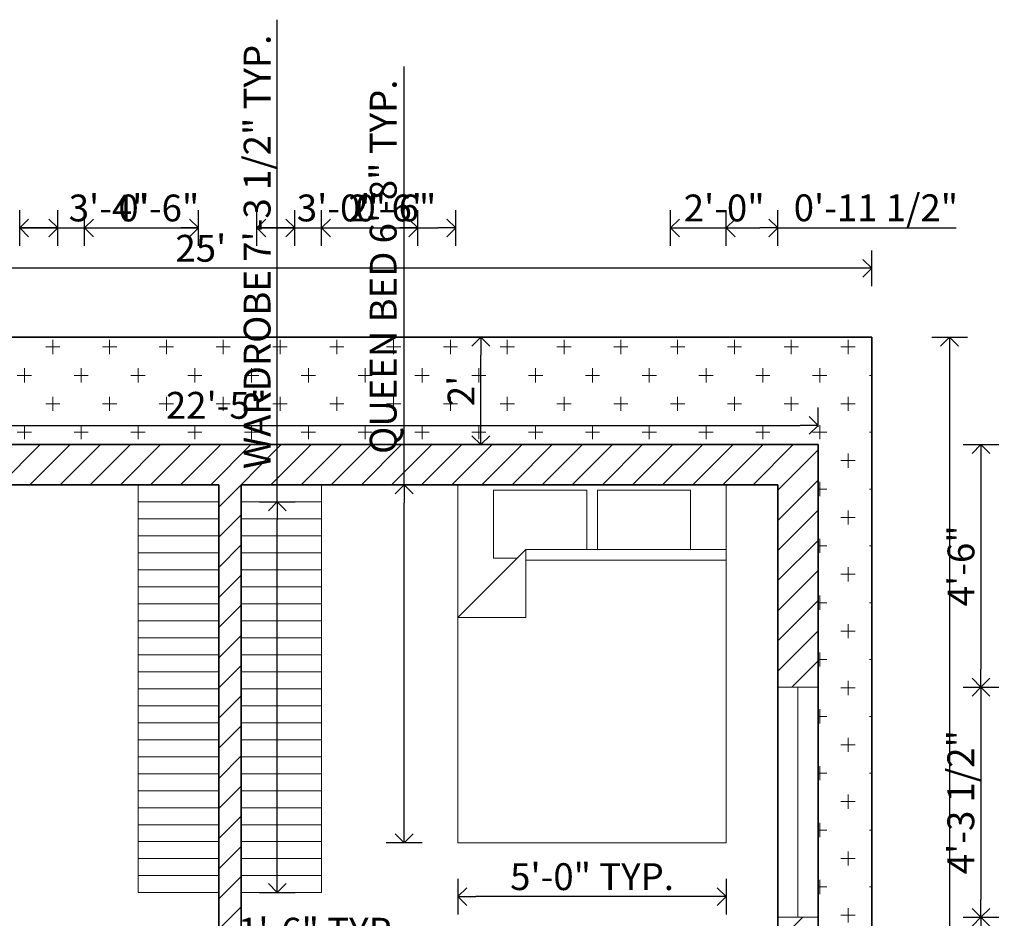
# Model space of a CAD drawing. Units: inches. Extents: x 686 to 1065, y 83 to 664.
# Tile 5 of 5: x 833 to 1053, y 463 to 664. Entities that reach past the tile are written whole.
import ezdxf

# ---------------------------------------------------------------- set-up
doc = ezdxf.new("R2010")
doc.units = ezdxf.units.IN
for name, color, linetype, lineweight in [('A-ANNO-DIMS', 2, 'Continuous', 18), ('A-FLOR-CABN', 8, 'Continuous', 20), ('A-FURN', 8, 'Continuous', 18), ('A-GLAZ', 172, 'Continuous', 18), ('A-WALL', 7, 'Continuous', 35), ('A-WALL-PATT', 253, 'Continuous', 13), ('C-PROP', 7, 'Continuous', 35), ('L-SITE-PATT', 94, 'Continuous', 13)]:
    doc.layers.add(name, color=color, linetype=linetype, lineweight=lineweight)
doc.styles.get("Standard").update_dxf_attribs({"font": 'arial.ttf'})
doc.dimstyles.new('ISO-25', dxfattribs={"dimtxt": 6, "dimasz": 4, "dimexe": 4, "dimexo": 4, "dimtad": 1, "dimdec": 1, "dimlunit": 3, "dimtxsty": 'Standard', "dimblk": 'OPEN90', "dimcen": 2.5, "dimadec": 0, "dimazin": 0, "dimtfac": 1, "dimtdec": 1, "dimtmove": 0, "dimatfit": 3, "dimfxl": 4, "dimfxlon": 1, "dimarcsym": 0})

# ---------------------------------------------------------------- blocks, each defined once
blk = doc.blocks.new('_Open90')
at = {"color": 0, "linetype": 'ByBlock', "lineweight": -2}
for p, q in [((0, 0), (-1, 0)), ((-0.5, 0.5), (0, 0)), ((0, 0), (-0.5, -0.5))]:
    blk.add_line(p, q, dxfattribs=at)
blk = doc.blocks.new('*D10')
at = {"layer": 'A-ANNO-DIMS', "color": 0, "lineweight": -2, "transparency": 16777216}
for p, q in [((939.95, 592.73), (931.95, 592.73)), ((935.95, 572.73), (935.95, 588.73)), ((939.95, 568.73), (931.95, 568.73))]:
    blk.add_line(p, q, dxfattribs=at)
at = {"layer": 'Defpoints', "color": 0, "transparency": 16777216}
for p in [(935.95, 592.73), (1011.37, 592.73), (1011.37, 568.73)]:
    blk.add_point(p, dxfattribs=at)
at = {"layer": 'A-ANNO-DIMS', "color": 0, "lineweight": -2, "transparency": 16777216, "xscale": 4, "yscale": 4, "zscale": 4}
for p, rotation in [((935.95, 592.73), 90), ((935.95, 568.73), 270)]:
    blk.add_blockref('_Open90', p, dxfattribs=dict(at, rotation=rotation))
at = {"layer": 'A-ANNO-DIMS', "color": 0, "transparency": 16777216, "insert": (932.32, 580.73), "char_height": 6, "attachment_point": 5, "rotation": 90}
blk.add_mtext("2'", dxfattribs=at)
blk = doc.blocks.new('*D11')
at = {"layer": 'A-ANNO-DIMS', "color": 0, "lineweight": -2, "transparency": 16777216}
for p, q in [((742.37, 572.73), (742.37, 577.04)), ((1011.37, 572.73), (1011.37, 577.04)), ((746.37, 573.04), (1007.37, 573.04))]:
    blk.add_line(p, q, dxfattribs=at)
at = {"layer": 'Defpoints', "color": 0, "transparency": 16777216}
for p in [(1011.37, 573.04), (742.37, 568.73), (1011.37, 568.73)]:
    blk.add_point(p, dxfattribs=at)
at = {"layer": 'A-ANNO-DIMS', "color": 0, "lineweight": -2, "transparency": 16777216, "xscale": 4, "yscale": 4, "zscale": 4, "rotation": 180}
blk.add_blockref('_Open90', (742.37, 573.04), dxfattribs=at)
at = {"layer": 'A-ANNO-DIMS', "color": 0, "lineweight": -2, "transparency": 16777216, "xscale": 4, "yscale": 4, "zscale": 4}
blk.add_blockref('_Open90', (1011.37, 573.04), dxfattribs=at)
at = {"layer": 'A-ANNO-DIMS', "color": 0, "transparency": 16777216, "insert": (876.87, 576.73), "char_height": 6, "attachment_point": 5}
blk.add_mtext('22\'-5"', dxfattribs=at)
blk = doc.blocks.new('Bed - Queen')
for p, q in [((0, -80.00003), (0, 0)), ((0, 0), (59.99999, 0)), ((59.99999, 0), (59.99999, -80.00003)), ((7.99999, -1.2), (28.79998, -1.2)), ((7.99999, -14.4), (7.99999, -1.2)), ((28.79998, -1.2), (28.79998, -14.4)), ((31.19999, -1.2), (51.99999, -1.2)), ((31.19999, -14.4), (31.19999, -1.2)), ((51.99999, -1.2), (51.99999, -16.4)), ((0, -14.4), (44.8, -14.4)), ((59.99999, -29.6), (44.8, -14.4)), ((44.8, -14.4), (44.8, -29.6)), ((44.8, -16.8), (0, -16.8)), ((51.99999, -16.4), (46.79936, -16.4)), ((44.8, -29.6), (59.99999, -29.6)), ((59.99999, -80.00003), (0, -80.00003))]:
    blk.add_line(p, q)
blk = doc.blocks.new('*D17')
at = {"layer": 'A-ANNO-DIMS', "color": 0, "lineweight": -2, "transparency": 16777216}
for p, q in [((723.37, 604.13), (723.37, 612.13)), ((1023.37, 604.13), (1023.37, 612.13)), ((1019.37, 608.13), (727.37, 608.13))]:
    blk.add_line(p, q, dxfattribs=at)
at = {"layer": 'Defpoints', "color": 0, "transparency": 16777216}
for p in [(723.37, 608.13), (723.37, 592.73), (1023.37, 592.73)]:
    blk.add_point(p, dxfattribs=at)
at = {"layer": 'A-ANNO-DIMS', "color": 0, "lineweight": -2, "transparency": 16777216, "xscale": 4, "yscale": 4, "zscale": 4, "rotation": 180}
blk.add_blockref('_Open90', (723.37, 608.13), dxfattribs=at)
at = {"layer": 'A-ANNO-DIMS', "color": 0, "lineweight": -2, "transparency": 16777216, "xscale": 4, "yscale": 4, "zscale": 4}
blk.add_blockref('_Open90', (1023.37, 608.13), dxfattribs=at)
at = {"layer": 'A-ANNO-DIMS', "color": 0, "transparency": 16777216, "insert": (873.37, 611.82), "char_height": 6, "attachment_point": 5}
blk.add_mtext("25'", dxfattribs=at)
blk = doc.blocks.new('*D8')
at = {"layer": 'A-ANNO-DIMS', "color": 0, "lineweight": -2, "transparency": 16777216}
for p, q in [((1036.76, 592.73), (1044.76, 592.73)), ((1040.76, 588.73), (1040.76, 164.73)), ((1036.76, 160.73), (1044.76, 160.73))]:
    blk.add_line(p, q, dxfattribs=at)
at = {"layer": 'Defpoints', "color": 0, "transparency": 16777216}
for p in [(1023.37, 592.73), (1023.37, 160.73), (1040.76, 160.73)]:
    blk.add_point(p, dxfattribs=at)
at = {"layer": 'A-ANNO-DIMS', "color": 0, "lineweight": -2, "transparency": 16777216, "xscale": 4, "yscale": 4, "zscale": 4}
for p, rotation in [((1040.76, 592.73), 90), ((1040.76, 160.73), 270)]:
    blk.add_blockref('_Open90', p, dxfattribs=dict(at, rotation=rotation))
at = {"layer": 'A-ANNO-DIMS', "color": 0, "transparency": 16777216, "insert": (1037.07, 376.73), "char_height": 6, "attachment_point": 5, "rotation": 90}
blk.add_mtext("36'", dxfattribs=at)
blk = doc.blocks.new('WARDROBE-SLATTED-RACK')
for p, q in [((0, 87.3), (18, 87.3)), ((0, 83.5), (18, 83.5)), ((0, 79.71), (18, 79.71)), ((0, 75.91), (18, 75.91)), ((0, 72.12), (18, 72.12)), ((0, 68.32), (18, 68.32)), ((0, 64.53), (18, 64.53)), ((0, 60.73), (18, 60.73)), ((0, 56.93), (18, 56.93)), ((0, 53.14), (18, 53.14)), ((0, 49.34), (18, 49.34)), ((0, 45.55), (18, 45.55)), ((0, 41.75), (18, 41.75)), ((0, 37.96), (18, 37.96)), ((0, 34.16), (18, 34.16)), ((0, 30.37), (18, 30.37)), ((0, 26.57), (18, 26.57)), ((0, 22.77), (18, 22.77)), ((0, 18.98), (18, 18.98)), ((0, 15.18), (18, 15.18)), ((0, 11.39), (18, 11.39)), ((0, 7.59), (18, 7.59)), ((0, 3.8), (18, 3.8)), ((6, 0), (0, 0)), ((18, 0), (6, 0))]:
    blk.add_line(p, q)
blk = doc.blocks.new('*D26')
at = {"layer": 'A-ANNO-DIMS', "color": 0, "lineweight": -2, "transparency": 16777216}
for p, q in [((918.83, 559.73), (918.83, 653.24)), ((922.83, 559.73), (914.83, 559.73)), ((918.83, 483.73), (918.83, 555.73)), ((922.83, 479.73), (914.83, 479.73))]:
    blk.add_line(p, q, dxfattribs=at)
at = {"layer": 'Defpoints', "color": 0, "transparency": 16777216}
for p in [(918.83, 559.73), (930.83, 559.73), (930.83, 479.73)]:
    blk.add_point(p, dxfattribs=at)
at = {"layer": 'A-ANNO-DIMS', "color": 0, "lineweight": -2, "transparency": 16777216, "xscale": 4, "yscale": 4, "zscale": 4}
for p, rotation in [((918.83, 559.73), 90), ((918.83, 479.73), 270)]:
    blk.add_blockref('_Open90', p, dxfattribs=dict(at, rotation=rotation))
at = {"layer": 'A-ANNO-DIMS', "color": 0, "transparency": 16777216, "insert": (914.92, 608.48), "char_height": 6, "attachment_point": 5, "rotation": 90}
blk.add_mtext('QUEEN BED 6\'-8" TYP.', dxfattribs=at)
blk = doc.blocks.new('*D27')
at = {"layer": 'A-ANNO-DIMS', "color": 0, "lineweight": -2, "transparency": 16777216}
for p, q in [((930.83, 471.73), (930.83, 463.73)), ((990.83, 471.73), (990.83, 463.73)), ((986.83, 467.73), (934.83, 467.73))]:
    blk.add_line(p, q, dxfattribs=at)
at = {"layer": 'Defpoints', "color": 0, "transparency": 16777216}
for p in [(930.83, 479.73), (990.83, 479.73), (930.83, 467.73)]:
    blk.add_point(p, dxfattribs=at)
at = {"layer": 'A-ANNO-DIMS', "color": 0, "lineweight": -2, "transparency": 16777216, "xscale": 4, "yscale": 4, "zscale": 4, "rotation": 180}
blk.add_blockref('_Open90', (930.83, 467.73), dxfattribs=at)
at = {"layer": 'A-ANNO-DIMS', "color": 0, "lineweight": -2, "transparency": 16777216, "xscale": 4, "yscale": 4, "zscale": 4}
blk.add_blockref('_Open90', (990.83, 467.73), dxfattribs=at)
at = {"layer": 'A-ANNO-DIMS', "color": 0, "transparency": 16777216, "insert": (960.83, 471.42), "char_height": 6, "attachment_point": 5}
blk.add_mtext('5\'-0" TYP.', dxfattribs=at)
blk = doc.blocks.new('*D28')
at = {"layer": 'A-ANNO-DIMS', "color": 0, "lineweight": -2, "transparency": 16777216}
for p, q in [((890.47, 555.93), (890.47, 663.68)), ((886.47, 555.93), (894.47, 555.93)), ((890.47, 472.63), (890.47, 551.93)), ((886.47, 468.63), (894.47, 468.63))]:
    blk.add_line(p, q, dxfattribs=at)
at = {"layer": 'Defpoints', "color": 0, "transparency": 16777216}
for p in [(877.37, 555.93), (890.47, 555.93), (877.37, 468.63)]:
    blk.add_point(p, dxfattribs=at)
at = {"layer": 'A-ANNO-DIMS', "color": 0, "lineweight": -2, "transparency": 16777216, "xscale": 4, "yscale": 4, "zscale": 4}
for p, rotation in [((890.47, 555.93), 90), ((890.47, 468.63), 270)]:
    blk.add_blockref('_Open90', p, dxfattribs=dict(at, rotation=rotation))
at = {"layer": 'A-ANNO-DIMS', "color": 0, "transparency": 16777216, "insert": (886.73, 611.8), "char_height": 6, "attachment_point": 5, "rotation": 90}
blk.add_mtext('WARDROBE 7\'-3 1/2" TYP.', dxfattribs=at)
blk = doc.blocks.new('*D29')
at = {"layer": 'A-ANNO-DIMS', "color": 0, "lineweight": -2, "transparency": 16777216}
for p, q in [((859.37, 459.54), (859.37, 451.54)), ((877.37, 459.54), (877.37, 451.54)), ((863.37, 455.54), (873.37, 455.54)), ((877.37, 455.54), (918.63, 455.54))]:
    blk.add_line(p, q, dxfattribs=at)
at = {"layer": 'Defpoints', "color": 0, "transparency": 16777216}
for p in [(859.37, 468.63), (877.37, 468.63), (877.37, 455.54)]:
    blk.add_point(p, dxfattribs=at)
at = {"layer": 'A-ANNO-DIMS', "color": 0, "lineweight": -2, "transparency": 16777216, "xscale": 4, "yscale": 4, "zscale": 4, "rotation": 180}
blk.add_blockref('_Open90', (859.37, 455.54), dxfattribs=at)
at = {"layer": 'A-ANNO-DIMS', "color": 0, "lineweight": -2, "transparency": 16777216, "xscale": 4, "yscale": 4, "zscale": 4}
blk.add_blockref('_Open90', (877.37, 455.54), dxfattribs=at)
at = {"layer": 'A-ANNO-DIMS', "color": 0, "transparency": 16777216, "insert": (900, 459.23), "char_height": 6, "attachment_point": 5}
blk.add_mtext('1\'-6" TYP.', dxfattribs=at)
blk = doc.blocks.new('*D46')
at = {"layer": 'A-ANNO-DIMS', "color": 0, "lineweight": -2, "transparency": 16777216}
for p, q in [((1043.78, 568.73), (1051.78, 568.73)), ((1047.78, 564.73), (1047.78, 518.56)), ((1043.78, 514.56), (1051.78, 514.56))]:
    blk.add_line(p, q, dxfattribs=at)
at = {"layer": 'Defpoints', "color": 0, "transparency": 16777216}
for p in [(1011.37, 568.73), (1011.37, 514.56), (1047.78, 514.56)]:
    blk.add_point(p, dxfattribs=at)
at = {"layer": 'A-ANNO-DIMS', "color": 0, "lineweight": -2, "transparency": 16777216, "xscale": 4, "yscale": 4, "zscale": 4}
for p, rotation in [((1047.78, 568.73), 90), ((1047.78, 514.56), 270)]:
    blk.add_blockref('_Open90', p, dxfattribs=dict(at, rotation=rotation))
at = {"layer": 'A-ANNO-DIMS', "color": 0, "transparency": 16777216, "insert": (1044.09, 541.65), "char_height": 6, "attachment_point": 5, "rotation": 90}
blk.add_mtext('4\'-6"', dxfattribs=at)
blk = doc.blocks.new('*D47')
at = {"layer": 'A-ANNO-DIMS', "color": 0, "lineweight": -2, "transparency": 16777216}
for p, q in [((1043.78, 514.56), (1051.78, 514.56)), ((1047.78, 510.56), (1047.78, 467.11)), ((1043.78, 463.11), (1051.78, 463.11))]:
    blk.add_line(p, q, dxfattribs=at)
at = {"layer": 'Defpoints', "color": 0, "transparency": 16777216}
for p in [(1011.37, 514.56), (1011.37, 463.11), (1047.78, 463.11)]:
    blk.add_point(p, dxfattribs=at)
at = {"layer": 'A-ANNO-DIMS', "color": 0, "lineweight": -2, "transparency": 16777216, "xscale": 4, "yscale": 4, "zscale": 4}
for p, rotation in [((1047.78, 514.56), 90), ((1047.78, 463.11), 270)]:
    blk.add_blockref('_Open90', p, dxfattribs=dict(at, rotation=rotation))
at = {"layer": 'A-ANNO-DIMS', "color": 0, "transparency": 16777216, "insert": (1044.05, 488.84), "char_height": 6, "attachment_point": 5, "rotation": 90}
blk.add_mtext('4\'-3 1/2"', dxfattribs=at)
blk = doc.blocks.new('*D48')
at = {"layer": 'A-ANNO-DIMS', "color": 0, "lineweight": -2, "transparency": 16777216}
for p, q in [((1043.78, 463.11), (1051.78, 463.11)), ((1047.78, 459.11), (1047.78, 367.95)), ((1043.78, 363.95), (1051.78, 363.95))]:
    blk.add_line(p, q, dxfattribs=at)
at = {"layer": 'Defpoints', "color": 0, "transparency": 16777216}
for p in [(1011.37, 463.11), (1011.37, 363.95), (1047.78, 363.95)]:
    blk.add_point(p, dxfattribs=at)
at = {"layer": 'A-ANNO-DIMS', "color": 0, "lineweight": -2, "transparency": 16777216, "xscale": 4, "yscale": 4, "zscale": 4}
for p, rotation in [((1047.78, 463.11), 90), ((1047.78, 363.95), 270)]:
    blk.add_blockref('_Open90', p, dxfattribs=dict(at, rotation=rotation))
at = {"layer": 'A-ANNO-DIMS', "color": 0, "transparency": 16777216, "insert": (1044.09, 413.53), "char_height": 6, "attachment_point": 5, "rotation": 90}
blk.add_mtext('8\'-3"', dxfattribs=at)
blk = doc.blocks.new('*D54')
at = {"layer": 'A-ANNO-DIMS', "color": 0, "lineweight": -2, "transparency": 16777216}
for p, q in [((832.87, 613.14), (832.87, 621.14)), ((872.87, 613.14), (872.87, 621.14)), ((836.87, 617.14), (868.87, 617.14))]:
    blk.add_line(p, q, dxfattribs=at)
at = {"layer": 'Defpoints', "color": 0, "transparency": 16777216}
for p in [(872.87, 617.14), (832.87, 415.73), (872.87, 415.73)]:
    blk.add_point(p, dxfattribs=at)
at = {"layer": 'A-ANNO-DIMS', "color": 0, "lineweight": -2, "transparency": 16777216, "xscale": 4, "yscale": 4, "zscale": 4, "rotation": 180}
blk.add_blockref('_Open90', (832.87, 617.14), dxfattribs=at)
at = {"layer": 'A-ANNO-DIMS', "color": 0, "lineweight": -2, "transparency": 16777216, "xscale": 4, "yscale": 4, "zscale": 4}
blk.add_blockref('_Open90', (872.87, 617.14), dxfattribs=at)
at = {"layer": 'A-ANNO-DIMS', "color": 0, "transparency": 16777216, "insert": (852.87, 620.83), "char_height": 6, "attachment_point": 5}
blk.add_mtext('3\'-4"', dxfattribs=at)
blk = doc.blocks.new('*D55')
at = {"layer": 'A-ANNO-DIMS', "color": 0, "lineweight": -2, "transparency": 16777216}
for p, q in [((885.87, 613.14), (885.87, 621.14)), ((921.87, 613.14), (921.87, 621.14)), ((889.87, 617.14), (917.87, 617.14))]:
    blk.add_line(p, q, dxfattribs=at)
at = {"layer": 'Defpoints', "color": 0, "transparency": 16777216}
for p in [(921.87, 617.14), (885.87, 415.73), (921.87, 415.73)]:
    blk.add_point(p, dxfattribs=at)
at = {"layer": 'A-ANNO-DIMS', "color": 0, "lineweight": -2, "transparency": 16777216, "xscale": 4, "yscale": 4, "zscale": 4, "rotation": 180}
blk.add_blockref('_Open90', (885.87, 617.14), dxfattribs=at)
at = {"layer": 'A-ANNO-DIMS', "color": 0, "lineweight": -2, "transparency": 16777216, "xscale": 4, "yscale": 4, "zscale": 4}
blk.add_blockref('_Open90', (921.87, 617.14), dxfattribs=at)
at = {"layer": 'A-ANNO-DIMS', "color": 0, "transparency": 16777216, "insert": (903.87, 620.83), "char_height": 6, "attachment_point": 5}
blk.add_mtext('3\'-0"', dxfattribs=at)
blk = doc.blocks.new('*D56')
at = {"layer": 'A-ANNO-DIMS', "color": 0, "lineweight": -2, "transparency": 16777216}
for p, q in [((900.37, 613.14), (900.37, 621.14)), ((930.37, 613.14), (930.37, 621.14)), ((904.37, 617.14), (926.37, 617.14))]:
    blk.add_line(p, q, dxfattribs=at)
at = {"layer": 'Defpoints', "color": 0, "transparency": 16777216}
for p in [(930.37, 617.14), (900.37, 246.73), (930.37, 246.73)]:
    blk.add_point(p, dxfattribs=at)
at = {"layer": 'A-ANNO-DIMS', "color": 0, "lineweight": -2, "transparency": 16777216, "xscale": 4, "yscale": 4, "zscale": 4, "rotation": 180}
blk.add_blockref('_Open90', (900.37, 617.14), dxfattribs=at)
at = {"layer": 'A-ANNO-DIMS', "color": 0, "lineweight": -2, "transparency": 16777216, "xscale": 4, "yscale": 4, "zscale": 4}
blk.add_blockref('_Open90', (930.37, 617.14), dxfattribs=at)
at = {"layer": 'A-ANNO-DIMS', "color": 0, "transparency": 16777216, "insert": (915.37, 620.83), "char_height": 6, "attachment_point": 5}
blk.add_mtext('2\'-6"', dxfattribs=at)
blk = doc.blocks.new('*D66')
at = {"layer": 'A-ANNO-DIMS', "color": 0, "lineweight": -2, "transparency": 16777216}
for p, q in [((894.37, 613.14), (894.37, 621.14)), ((900.37, 613.14), (900.37, 621.14)), ((890.37, 617.14), (886.37, 617.14)), ((894.37, 617.14), (900.37, 617.14)), ((904.37, 617.14), (925.57, 617.14))]:
    blk.add_line(p, q, dxfattribs=at)
at = {"layer": 'Defpoints', "color": 0, "transparency": 16777216}
for p in [(900.37, 617.14), (894.37, 241.73), (900.37, 241.73)]:
    blk.add_point(p, dxfattribs=at)
at = {"layer": 'A-ANNO-DIMS', "color": 0, "lineweight": -2, "transparency": 16777216, "xscale": 4, "yscale": 4, "zscale": 4}
blk.add_blockref('_Open90', (894.37, 617.14), dxfattribs=at)
at = {"layer": 'A-ANNO-DIMS', "color": 0, "lineweight": -2, "transparency": 16777216, "xscale": 4, "yscale": 4, "zscale": 4, "rotation": 180}
blk.add_blockref('_Open90', (900.37, 617.14), dxfattribs=at)
at = {"layer": 'A-ANNO-DIMS', "color": 0, "transparency": 16777216, "insert": (916.97, 620.83), "char_height": 6, "attachment_point": 5}
blk.add_mtext('0\'-6"', dxfattribs=at)
blk = doc.blocks.new('*D69')
at = {"layer": 'A-ANNO-DIMS', "color": 0, "lineweight": -2, "transparency": 16777216}
for p, q in [((978.37, 613.14), (978.37, 621.14)), ((1002.37, 613.14), (1002.37, 621.14)), ((982.37, 617.14), (998.37, 617.14))]:
    blk.add_line(p, q, dxfattribs=at)
at = {"layer": 'Defpoints', "color": 0, "transparency": 16777216}
for p in [(1002.37, 617.14), (978.37, 241.73), (1002.37, 241.73)]:
    blk.add_point(p, dxfattribs=at)
at = {"layer": 'A-ANNO-DIMS', "color": 0, "lineweight": -2, "transparency": 16777216, "xscale": 4, "yscale": 4, "zscale": 4, "rotation": 180}
blk.add_blockref('_Open90', (978.37, 617.14), dxfattribs=at)
at = {"layer": 'A-ANNO-DIMS', "color": 0, "lineweight": -2, "transparency": 16777216, "xscale": 4, "yscale": 4, "zscale": 4}
blk.add_blockref('_Open90', (1002.37, 617.14), dxfattribs=at)
at = {"layer": 'A-ANNO-DIMS', "color": 0, "transparency": 16777216, "insert": (990.37, 620.83), "char_height": 6, "attachment_point": 5}
blk.add_mtext('2\'-0"', dxfattribs=at)
blk = doc.blocks.new('*D75')
at = {"layer": 'A-ANNO-DIMS', "color": 0, "lineweight": -2, "transparency": 16777216}
for p, q in [((841.37, 613.14), (841.37, 621.14)), ((847.37, 613.14), (847.37, 621.14)), ((837.37, 617.14), (833.37, 617.14)), ((841.37, 617.14), (847.37, 617.14)), ((851.37, 617.14), (872.57, 617.14))]:
    blk.add_line(p, q, dxfattribs=at)
at = {"layer": 'Defpoints', "color": 0, "transparency": 16777216}
for p in [(847.37, 617.14), (841.37, 169.73), (847.37, 169.73)]:
    blk.add_point(p, dxfattribs=at)
at = {"layer": 'A-ANNO-DIMS', "color": 0, "lineweight": -2, "transparency": 16777216, "xscale": 4, "yscale": 4, "zscale": 4}
blk.add_blockref('_Open90', (841.37, 617.14), dxfattribs=at)
at = {"layer": 'A-ANNO-DIMS', "color": 0, "lineweight": -2, "transparency": 16777216, "xscale": 4, "yscale": 4, "zscale": 4, "rotation": 180}
blk.add_blockref('_Open90', (847.37, 617.14), dxfattribs=at)
at = {"layer": 'A-ANNO-DIMS', "color": 0, "transparency": 16777216, "insert": (863.97, 620.83), "char_height": 6, "attachment_point": 5}
blk.add_mtext('0\'-6"', dxfattribs=at)
blk = doc.blocks.new('*D77')
at = {"layer": 'A-ANNO-DIMS', "color": 0, "lineweight": -2, "transparency": 16777216}
for p, q in [((990.83, 613.14), (990.83, 621.14)), ((1002.37, 613.14), (1002.37, 621.14)), ((994.83, 617.14), (998.37, 617.14)), ((1002.37, 617.14), (1042.21, 617.14))]:
    blk.add_line(p, q, dxfattribs=at)
at = {"layer": 'Defpoints', "color": 0, "transparency": 16777216}
for p in [(1002.37, 617.14), (990.83, 559.73), (1002.37, 559.73)]:
    blk.add_point(p, dxfattribs=at)
at = {"layer": 'A-ANNO-DIMS', "color": 0, "lineweight": -2, "transparency": 16777216, "xscale": 4, "yscale": 4, "zscale": 4, "rotation": 180}
blk.add_blockref('_Open90', (990.83, 617.14), dxfattribs=at)
at = {"layer": 'A-ANNO-DIMS', "color": 0, "lineweight": -2, "transparency": 16777216, "xscale": 4, "yscale": 4, "zscale": 4}
blk.add_blockref('_Open90', (1002.37, 617.14), dxfattribs=at)
at = {"layer": 'A-ANNO-DIMS', "color": 0, "transparency": 16777216, "insert": (1024.29, 620.87), "char_height": 6, "attachment_point": 5}
blk.add_mtext('0\'-11 1/2"', dxfattribs=at)

msp = doc.modelspace()

# ---------------------------------------------------------------- hatches: boundary and pattern name
at = {"layer": 'A-WALL-PATT'}
h = msp.add_hatch(dxfattribs=at)
h.set_pattern_fill('ANSI31', color=256, scale=1.5)
h.set_pattern_definition([(45, (464.028, 0), (-3.367596, 3.367596), [])])
h.paths.add_polyline_path([(1011.37, 568.73), (742.37, 568.73), (742.37, 499.41), (751.37, 499.41), (751.37, 559.73), (877.37, 559.73), (877.37, 415.73), (872.87, 415.73), (872.87, 410.73), (885.87, 410.73), (885.87, 415.73), (882.37, 415.73), (882.37, 559.73), (1002.37, 559.73), (1002.37, 514.56), (1011.37, 514.56)])
h.paths.add_polyline_path([(832.87, 415.73), (751.37, 415.73), (751.37, 448.47), (742.37, 448.47), (742.37, 397.23), (751.37, 397.23), (751.37, 410.73), (823.37, 410.73), (823.37, 404.73), (828.37, 404.73), (828.37, 410.73), (832.87, 410.73)])
h.paths.add_polyline_path([(751.37, 357.73), (828.37, 357.73), (828.37, 372.73), (823.37, 372.73), (823.37, 362.73), (751.37, 362.73), (751.37, 376.23), (742.37, 376.23), (742.37, 112.73), (751.37, 112.73)])
h.paths.add_polyline_path([(845.37, 160.73), (847.37, 160.73), (847.37, 169.73), (841.37, 169.73), (841.37, 246.73), (836.37, 246.73), (836.37, 117.73), (807.43, 117.73), (807.43, 112.73), (845.37, 112.73)])
h.paths.add_polyline_path([(920.89, 169.73), (904.39, 169.73), (894.37, 169.73), (894.37, 241.73), (900.37, 241.73), (900.37, 246.73), (889.37, 246.73), (889.37, 169.73), (883.37, 169.73), (883.37, 160.73), (920.89, 160.73)])
h.paths.add_polyline_path([(1011.37, 196.2), (1002.37, 196.2), (1002.37, 169.73), (966.91, 169.73), (966.91, 160.73), (1011.37, 160.73)])
h.paths.add_polyline_path([(1011.37, 307.98), (1002.37, 307.98), (1002.37, 232.2), (1011.37, 232.2)])
h.paths.add_polyline_path([(1011.37, 463.11), (1002.37, 463.11), (1002.37, 415.73), (921.87, 415.73), (921.87, 410.73), (1002.37, 410.73), (1002.37, 363.95), (1011.37, 363.95)])
h.paths.add_polyline_path([(781.1, 117.73), (751.37, 117.73), (751.37, 112.73), (781.1, 112.73)], flags=17)
at = {"layer": 'L-SITE-PATT'}
h = msp.add_hatch(dxfattribs=at)
h.set_pattern_fill('CROSS', color=256)
h.set_pattern_definition([(0, (464.028, 0), (6.35, 6.35), [3.175, -9.525]), (90, (465.6154, -1.5875), (-6.35, 6.35), [3.175, -9.525])])
h.paths.add_polyline_path([(742.37, 568.73), (1011.37, 568.73), (1011.37, 160.73), (1023.37, 160.73), (1023.37, 592.73), (723.37, 592.73), (723.37, 112.73), (742.37, 112.73)])
h.paths.add_polyline_path([(1012.48, 266.46), (1021.74, 266.46), (1021.74, 278.82), (1012.48, 278.82)], flags=24)
h.paths.add_polyline_path([(938.61, 576.17), (938.61, 585.43), (926.24, 585.43), (926.24, 576.17)], flags=24)
h.paths.add_polyline_path([(864.77, 570.5), (889.12, 570.5), (889.12, 582.86), (864.77, 582.86)], flags=24)
h.paths.add_polyline_path([(722.77, 199.16), (742.46, 199.16), (742.46, 211.52), (722.77, 211.52)], flags=9)

# ---------------------------------------------------------------- linework, layer by layer
at = {"layer": 'A-FLOR-CABN'}
for p, q in [((859.37, 468.63), (859.37, 559.73)), ((900.37, 468.63), (900.37, 559.73))]:
    msp.add_line(p, q, dxfattribs=at)
at = {"layer": 'A-GLAZ'}
for p, q in [((1002.37, 514.56), (1011.37, 514.56)), ((1006.87, 514.56), (1006.87, 463.11)), ((1002.37, 463.11), (1011.37, 463.11))]:
    msp.add_line(p, q, dxfattribs=at)
at = {"layer": 'A-WALL'}
for p, q in [((1011.37, 568.73), (742.37, 568.73)), ((1011.37, 160.73), (1011.37, 568.73)), ((877.37, 559.73), (751.37, 559.73)), ((877.37, 559.73), (877.37, 415.73)), ((1002.37, 559.73), (882.37, 559.73)), ((882.37, 559.73), (882.37, 415.73)), ((1002.37, 415.73), (1002.37, 559.73))]:
    msp.add_line(p, q, dxfattribs=at)
at = {"layer": 'C-PROP'}
for p, q in [((1023.37, 592.73), (723.37, 592.73)), ((1023.37, 112.73), (1023.37, 592.73))]:
    msp.add_line(p, q, dxfattribs=at)

# ---------------------------------------------------------------- block references
at = {"layer": 'A-FLOR-CABN'}
for p in [(859.37, 468.63), (882.37, 468.63)]:
    msp.add_blockref('WARDROBE-SLATTED-RACK', p, dxfattribs=at)
at = {"layer": 'A-FURN', "xscale": -1}
msp.add_blockref('Bed - Queen', (990.83, 559.73), dxfattribs=at)

# ---------------------------------------------------------------- dimensions: what is measured, and where the dimension line sits
at = {"layer": 'A-ANNO-DIMS'}
for base, p1, p2, angle, text, picture, middle in [((890.47, 555.93), (877.37, 468.63), (877.37, 555.93), 90, 'WARDROBE <> TYP.', '*D28', (886.73, 611.8)), ((918.83, 559.73), (930.83, 479.73), (930.83, 559.73), 90, 'QUEEN BED <> TYP.', '*D26', (914.92, 608.48)), ((930.83, 467.73), (990.83, 479.73), (930.83, 479.73), 180, '<> TYP.', '*D27', (960.83, 471.42))]:
    dim = msp.add_linear_dim(base=base, p1=p1, p2=p2, angle=angle, text=text, dimstyle='ISO-25', override={"dimdec": 1, "dimlfac": 1, "dimrnd": 0, "dimzin": 1, "dimdsep": 46, "dimlunit": 4, "dimfrac": 2}, dxfattribs=at)
    dim.commit()
    dim.dimension.update_dxf_attribs({"geometry": picture, "text_midpoint": middle})
for base, p1, p2, override, picture, middle in [((1002.37, 617.14), (990.83, 559.73), (1002.37, 559.73), {"dimdec": 1, "dimlfac": 1, "dimrnd": 0, "dimzin": 1, "dimdsep": 46, "dimlunit": 4, "dimfrac": 2}, '*D77', (1024.29, 620.87)), ((872.87, 617.14), (832.87, 415.73), (872.87, 415.73), {"dimdec": 1, "dimlfac": 1, "dimrnd": 0, "dimzin": 1, "dimdsep": 46, "dimlunit": 4, "dimfrac": 2}, '*D54', (852.87, 620.83)), ((847.37, 617.14), (841.37, 169.73), (847.37, 169.73), {"dimdec": 1, "dimlfac": 1, "dimrnd": 0, "dimzin": 1, "dimdsep": 46, "dimlunit": 4, "dimfrac": 2}, '*D75', (863.97, 620.83)), ((921.87, 617.14), (885.87, 415.73), (921.87, 415.73), {"dimdec": 1, "dimlfac": 1, "dimrnd": 0, "dimzin": 1, "dimdsep": 46, "dimlunit": 4, "dimfrac": 2}, '*D55', (903.87, 620.83)), ((900.37, 617.14), (894.37, 241.73), (900.37, 241.73), {"dimdec": 1, "dimlfac": 1, "dimrnd": 0, "dimzin": 1, "dimdsep": 46, "dimlunit": 4, "dimfrac": 2}, '*D66', (916.97, 620.83)), ((930.37, 617.14), (900.37, 246.73), (930.37, 246.73), {"dimdec": 1, "dimlfac": 1, "dimrnd": 0, "dimzin": 1, "dimdsep": 46, "dimlunit": 4, "dimfrac": 2}, '*D56', (915.37, 620.83)), ((1002.37, 617.14), (978.37, 241.73), (1002.37, 241.73), {"dimdec": 1, "dimlfac": 1, "dimrnd": 0, "dimzin": 1, "dimdsep": 46, "dimlunit": 4, "dimfrac": 2}, '*D69', (990.37, 620.83)), ((723.37, 608.13), (1023.37, 592.73), (723.37, 592.73), {"dimclrd": 0, "dimclre": 0, "dimclrt": 0}, '*D17', (873.37, 611.82)), ((1011.37, 573.04), (742.37, 568.73), (1011.37, 568.73), {"dimclrd": 0, "dimclre": 0, "dimclrt": 0}, '*D11', (876.87, 576.73))]:
    dim = msp.add_linear_dim(base=base, p1=p1, p2=p2, dimstyle='ISO-25', override=override, dxfattribs=at)
    dim.commit()
    dim.dimension.update_dxf_attribs({"geometry": picture, "text_midpoint": middle})
for base, p1, p2, override, picture, middle in [((935.95, 592.73), (1011.37, 568.73), (1011.37, 592.73), {"dimclrd": 0, "dimclre": 0, "dimclrt": 0}, '*D10', (932.32, 580.73)), ((1040.76, 160.73), (1023.37, 592.73), (1023.37, 160.73), {"dimclrd": 0, "dimclre": 0, "dimclrt": 0}, '*D8', (1037.07, 376.73)), ((1047.78, 514.56), (1011.37, 568.73), (1011.37, 514.56), {"dimdec": 1, "dimlfac": 1, "dimrnd": 0, "dimzin": 1, "dimdsep": 46, "dimlunit": 4, "dimfrac": 2}, '*D46', (1044.09, 541.65)), ((1047.7813, 463.1132), (1011.3713, 514.5633), (1011.3713, 463.1132), {"dimdec": 1, "dimlfac": 1, "dimrnd": 0, "dimzin": 1, "dimdsep": 46, "dimlunit": 4, "dimfrac": 2}, '*D47', (1044.0519, 488.8383)), ((1047.78, 363.95), (1011.37, 463.11), (1011.37, 363.95), {"dimdec": 1, "dimlfac": 1, "dimrnd": 0, "dimzin": 1, "dimdsep": 46, "dimlunit": 4, "dimfrac": 2}, '*D48', (1044.09, 413.53))]:
    dim = msp.add_linear_dim(base=base, p1=p1, p2=p2, angle=90, dimstyle='ISO-25', override=override, dxfattribs=at)
    dim.commit()
    dim.dimension.update_dxf_attribs({"geometry": picture, "text_midpoint": middle})
dim = msp.add_linear_dim(base=(877.37, 455.54), p1=(859.37, 468.63), p2=(877.37, 468.63), text='<> TYP.', dimstyle='ISO-25', override={"dimdec": 1, "dimlfac": 1, "dimrnd": 0, "dimzin": 1, "dimdsep": 46, "dimlunit": 4, "dimfrac": 2}, dxfattribs=at)
dim.commit()
dim.dimension.update_dxf_attribs({"geometry": '*D29', "text_midpoint": (900, 459.23)})

doc.saveas('drawing.dxf')
